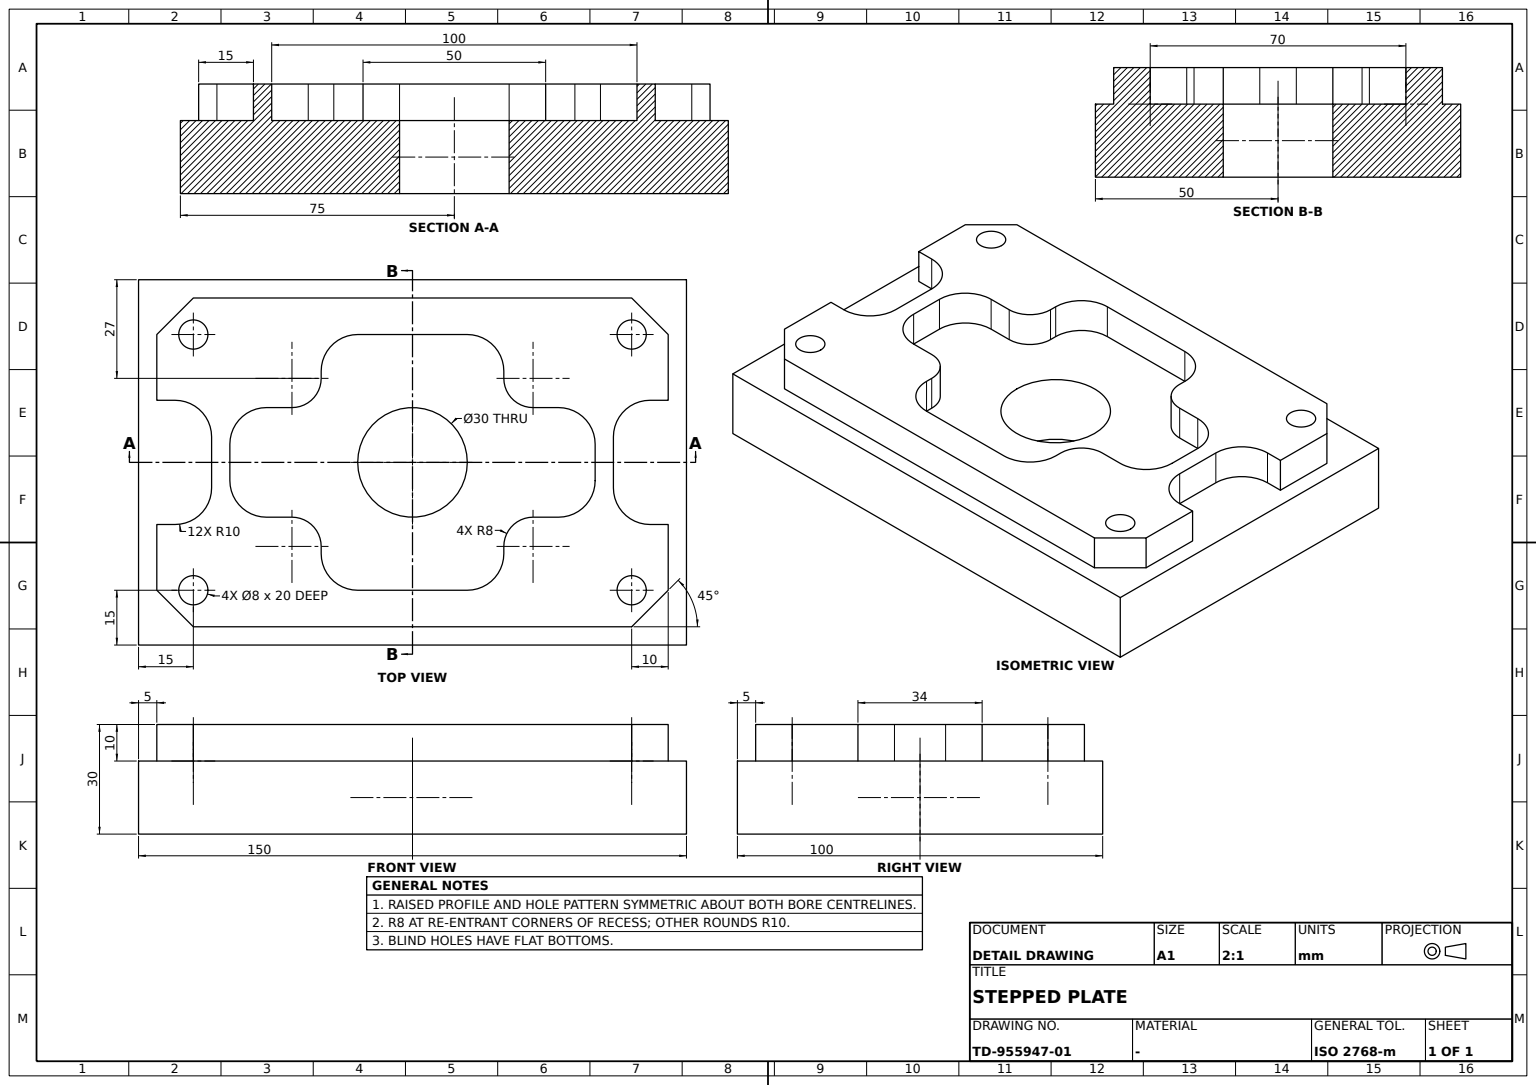
CATIA V5 part; units mm, degrees
sketch "Sketch1" plane through (0, 0, 0) normal (0, 0, 1) x (1, 0, 0)
  line L0 (75, 50) -> (75, -50)
  line L1 (75, -50) -> (-75, -50)
  line L2 (-75, -50) -> (-75, 50)
  line L3 (-75, 50) -> (75, 50)
  dimension "length L0" = 100
  dimension "length L3" = 150
  constraint vertical L0 y-axis
  constraint vertical L2 y-axis
  constraint horizontal L1 x-axis
  constraint horizontal L3 x-axis
  constraint equidistance L0 L2 origin
  constraint equidistance L1 L3 origin
extrude "Pad1" add sketch "Sketch1" along normal mid plane 20
sketch "Sketch2" plane through (0, 0, -10) normal (0, 0, -1) x (1, 0, 0)
  circle A0 centre (-60, -35) radius 4
  point P0 (-60, -35)
  circle A1 centre (-60, 35) radius 4
  point P1 (-60, 35)
  line L0 (-75, -50) -> (75, -50) construction
  line L1 (-75, 50) -> (-75, -50) construction
  line L2 (75, 50) -> (-75, 50) construction
  line L3 (-75, 50) -> (-75, -50) construction
  circle A2 centre (60, -35) radius 4
  circle A3 centre (60, 35) radius 4
  dimension "radius A0" = 4
  dimension "distance P0 L0" = 15
  dimension "distance P0 L1" = 15
  dimension "radius A1" = 4
  dimension "distance P1 L2" = 15
  dimension "distance L3 P1" = 15
  constraint symmetry A0 A2 y-axis
  constraint symmetry A1 A3 y-axis
extrude "Pocket1" cut sketch "Sketch2" against normal blind 20
sketch "Sketch3" plane through (0, 0, -10) normal (0, 0, -1) x (1, 0, 0)
  line L0 (50, 5) -> (50, -5)
  line L1 (40, -15) -> (33, -15)
  line L2 (-50, -5) -> (-50, 5)
  line L3 (-40, 15) -> (-33, 15)
  point P0 (50, 15)
  point P1 (50, -15)
  point P2 (-50, 15)
  line L4 (25, 25) -> (25, 23)
  line L5 (15, -35) -> (-15, -35)
  line L6 (-25, -25) -> (-25, -23)
  line L7 (-15, 35) -> (15, 35)
  point P3 (25, 35)
  point P4 (25, -35)
  point P5 (-25, 35)
  point P6 (-25, -15)
  line L8 (-25, 23) -> (-25, 25)
  line L9 (33, 15) -> (40, 15)
  line L10 (25, -23) -> (25, -25)
  line L11 (-33, -15) -> (-40, -15)
  arc A0 (-33, 15) -> (-25, 23) centre (-33, 23) ccw
  arc A1 (-33, -15) -> (-25, -23) centre (-33, -23) cw
  arc A2 (25, -23) -> (33, -15) centre (33, -23) cw
  arc A3 (25, 23) -> (33, 15) centre (33, 23) ccw
  arc A4 (-25, 25) -> (-15, 35) centre (-15, 25) cw
  arc A5 (15, 35) -> (25, 25) centre (15, 25) cw
  arc A6 (-50, 5) -> (-40, 15) centre (-40, 5) cw
  arc A7 (-50, -5) -> (-40, -15) centre (-40, -5) ccw
  arc A8 (-25, -25) -> (-15, -35) centre (-15, -25) ccw
  arc A9 (15, -35) -> (25, -25) centre (15, -25) ccw
  arc A10 (40, -15) -> (50, -5) centre (40, -5) ccw
  arc A11 (40, 15) -> (50, 5) centre (40, 5) cw
  dimension "distance P2 P0" = 100
  dimension "distance P3 P4" = 70
  dimension "radius A0" = 8
  dimension "radius A1" = 8
  dimension "radius A2" = 8
  dimension "radius A3" = 8
  dimension "distance P5 P3" = 50
  dimension "radius A4" = 10
  dimension "radius A5" = 10
  dimension "radius A6" = 10
  dimension "radius A7" = 10
  dimension "radius A8" = 10
  dimension "radius A9" = 10
  dimension "distance P0 P1" = 30
  dimension "radius A10" = 10
  dimension "radius A11" = 10
  constraint vertical L0 y-axis
  constraint vertical L2 y-axis
  constraint vertical L4 y-axis
  constraint vertical L6 y-axis
  constraint vertical L8 y-axis
  constraint vertical L10 y-axis
  constraint horizontal L1 x-axis
  constraint horizontal L3 x-axis
  constraint horizontal L5 x-axis
  constraint horizontal L7 x-axis
  constraint horizontal L9 x-axis
  constraint horizontal L11 x-axis
  constraint equidistance L0 L2 origin
  constraint equidistance L1 L3 origin
  constraint equidistance L4 L6 origin
  constraint equidistance L5 L7 origin
  constraint coincidence L1 P6
  constraint coincidence L6 L8
  constraint coincidence L3 L9
  constraint coincidence L4 L10
  constraint coincidence L1 L11
  constraint coincidence L11 P6
  constraint coincidence L6 P6
  constraint coincidence L8 P5
  constraint coincidence L7 P5
  constraint coincidence L7 P3
  constraint coincidence L4 P3
  constraint coincidence L2 P2
  constraint coincidence L3 P2
  constraint coincidence L5 P4
  constraint coincidence L10 P4
  constraint coincidence L1 P1
  constraint coincidence L0 P1
  constraint coincidence L9 P0
  constraint coincidence L0 P0
  constraint tangency A0 L3
  constraint tangency A0 L8
  constraint tangency A1 L11
  constraint tangency A1 L6
  constraint tangency A2 L10
  constraint tangency A2 L1
  constraint tangency A3 L4
  constraint tangency A3 L9
  constraint tangency A4 L8
  constraint tangency A4 L7
  constraint tangency A5 L7
  constraint tangency A5 L4
  constraint tangency A6 L2
  constraint tangency A6 L3
  constraint tangency A7 L2
  constraint tangency A7 L11
  constraint tangency A8 L6
  constraint tangency A8 L5
  constraint tangency A9 L5
  constraint tangency A9 L10
  constraint tangency A10 L1
  constraint tangency A10 L0
  constraint tangency A11 L9
  constraint tangency A11 L0
extrude "Pocket2" cut sketch "Sketch3" against normal blind 10
sketch "Sketch4" plane through (0, 0, -10) normal (0, 0, -1) x (1, 0, 0)
  line L0 (-75, 50) -> (-75, -50) construction
  line L1 (70, -50) -> (70, 50) construction
  line L2 (70, 45) -> (70, -45)
  line L3 (-75, -45) -> (75, -45) construction
  line L4 (70, -45) -> (-70, -45)
  line L5 (-70, 50) -> (-70, -50) construction
  line L6 (-70, -45) -> (-70, 45)
  line L7 (75, 45) -> (-75, 45) construction
  line L8 (-70, 45) -> (70, 45)
  point P0 (-70, 45)
  point P1 (-70, 45)
  point P2 (70, 45)
  point P3 (70, 45)
  point P4 (70, -45)
  point P5 (70, -45)
  point P6 (-70, -45)
  point P7 (-70, -45)
  dimension "distance L0 L5" = 5
  constraint coincidence L5 P0
  constraint coincidence L7 P1
  constraint coincidence L7 P2
  constraint coincidence L1 P3
  constraint coincidence L1 P4
  constraint coincidence L3 P5
  constraint coincidence L3 P6
  constraint coincidence L5 P7
  constraint coincidence P0 P1
  constraint coincidence P2 P3
  constraint coincidence P4 P5
  constraint coincidence P6 P7
extrude "Pocket3" cut sketch "Sketch4" against normal blind 10 flip side to cut
chamfer "Chamfer1" distance 10 angle 45 4 edges at (70, -45, -5) (70, 45, -5) (-70, 45, -5) (-70, -45, -5)
sketch "Sketch5" plane through (0, 0, -10) normal (0, 0, -1) x (1, 0, 0)
  point P0 (62.5, 0)
  line L0 (70, 17) -> (70, -17)
  line L1 (70, -17) -> (65, -17)
  line L2 (55, -7) -> (55, 7)
  line L3 (65, 17) -> (70, 17)
  point P1 (70, 17)
  point P2 (70, -17)
  point P3 (55, -17)
  point P4 (55, 17)
  line L4 (70, -45) -> (70, 45) construction
  arc A0 (55, -7) -> (65, -17) centre (65, -7) ccw
  point P5 (55, -7)
  point P6 (65, -17)
  arc A1 (55, 7) -> (65, 17) centre (65, 7) cw
  point P7 (55, 7)
  point P8 (65, 17)
  point P9 (-62.5, 0)
  point P10 (-70, 17)
  point P11 (-70, -17)
  point P12 (-55, -17)
  point P13 (-55, 17)
  point P14 (-55, -7)
  point P15 (-65, -17)
  point P16 (-55, 7)
  point P17 (-65, 17)
  line L5 (-70, 17) -> (-70, -17)
  line L6 (-70, -17) -> (-65, -17)
  line L7 (-55, -7) -> (-55, 7)
  line L8 (-65, 17) -> (-70, 17)
  arc A2 (-55, -7) -> (-65, -17) centre (-65, -7) cw
  arc A3 (-55, 7) -> (-65, 17) centre (-65, 7) ccw
  dimension "distance P3 P4" = 34
  dimension "distance P2 P3" = 15
  dimension "radius A0" = 10
  dimension "radius A1" = 10
  constraint coincidence P0 x-axis
  constraint coincidence L0 L4
  constraint coincidence L2 P3
  constraint coincidence L1 P3
  constraint coincidence L2 P4
  constraint coincidence L3 P4
  constraint vertical L0 y-axis
  constraint vertical L2 y-axis
  constraint horizontal L1 x-axis
  constraint horizontal L3 x-axis
  constraint equidistance L0 L2 P0
  constraint equidistance L1 L3 P0
  constraint tangency A0 L2
  constraint tangency A0 L1
  constraint tangency A1 L2
  constraint tangency A1 L3
  constraint symmetry L3 L1 x-axis
  constraint symmetry P0 P9 y-axis
  constraint symmetry P1 P10 y-axis
  constraint symmetry P2 P11 y-axis
  constraint symmetry P3 P12 y-axis
  constraint symmetry P4 P13 y-axis
  constraint symmetry P5 P14 y-axis
  constraint symmetry P6 P15 y-axis
  constraint symmetry P7 P16 y-axis
  constraint symmetry P8 P17 y-axis
  constraint symmetry L0 L5 y-axis
  constraint symmetry L1 L6 y-axis
  constraint symmetry L2 L7 y-axis
  constraint symmetry L3 L8 y-axis
  constraint symmetry A0 A2 y-axis
  constraint symmetry A1 A3 y-axis
extrude "Pocket4" cut sketch "Sketch5" against normal blind 10
sketch "Sketch6" plane through (0, 0, 10) normal (0, 0, 1) x (1, 0, 0)
  line L0 (-75, -50) -> (-75, 50)
  line L1 (-75, 50) -> (75, 50)
  line L2 (75, 50) -> (75, -50)
  line L3 (75, -50) -> (-75, -50)
extrude "Pad2" add sketch "Sketch6" along normal blind 10
sketch "Sketch7" plane through (0, 0, 0) normal (0, 0, -1) x (1, 0, 0)
  circle A0 centre (0, 0) radius 15
  dimension "radius A0" = 15
extrude "Pocket5" cut sketch "Sketch7" against normal through all
